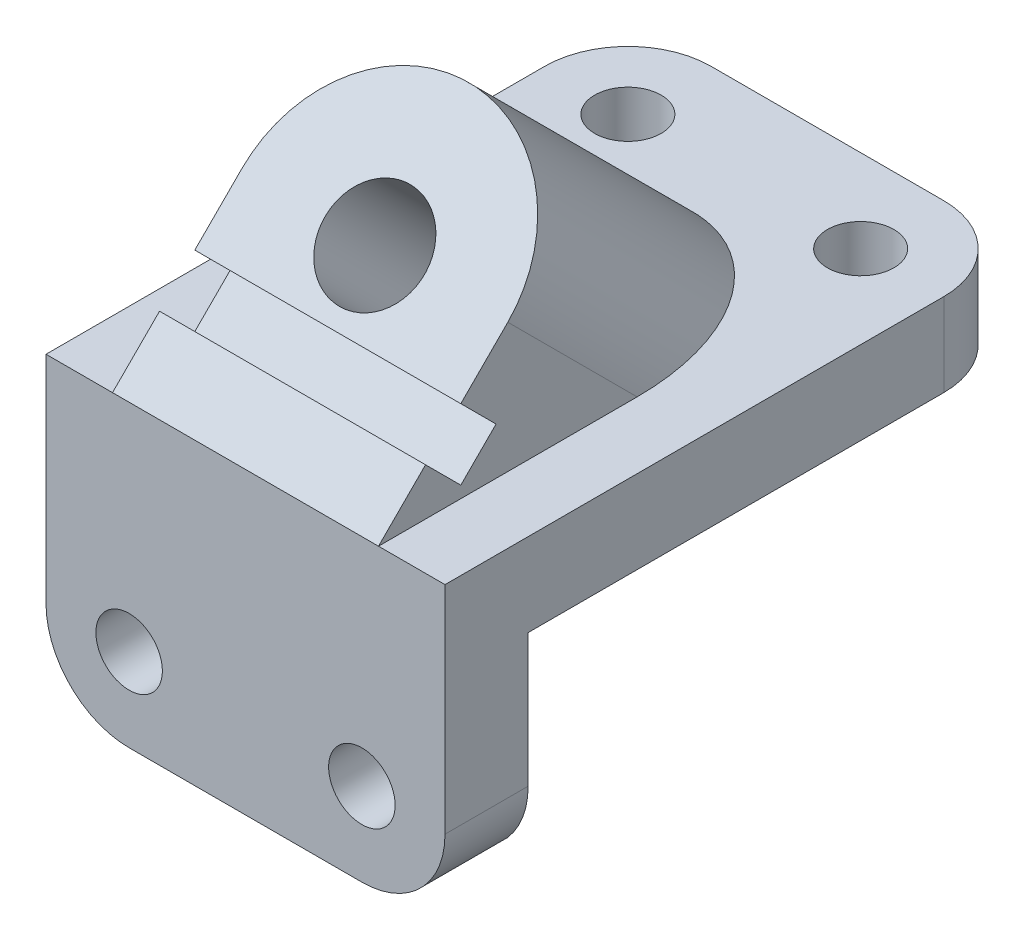
ISO-10303-21;
HEADER;
FILE_DESCRIPTION(('STEP AP214'),'2;1');
FILE_NAME('part.step','',(''),(''),'','','');
FILE_SCHEMA(('AUTOMOTIVE_DESIGN { 1 0 10303 214 1 1 1 1 }'));
ENDSEC;
DATA;
#1=APPLICATION_CONTEXT('core data for automotive mechanical design processes');
#2=APPLICATION_PROTOCOL_DEFINITION('international standard','automotive_design',2000,#1);
#3=PRODUCT_CONTEXT('',#1,'mechanical');
#4=PRODUCT('Part','Part','',(#3));
#5=PRODUCT_RELATED_PRODUCT_CATEGORY('part','',(#4));
#6=PRODUCT_DEFINITION_FORMATION('','',#4);
#7=PRODUCT_DEFINITION_CONTEXT('part definition',#1,'design');
#8=PRODUCT_DEFINITION('design','',#6,#7);
#9=PRODUCT_DEFINITION_SHAPE('','',#8);
#10=(LENGTH_UNIT() NAMED_UNIT(*) SI_UNIT(.MILLI.,.METRE.));
#11=(NAMED_UNIT(*) PLANE_ANGLE_UNIT() SI_UNIT($,.RADIAN.));
#12=(NAMED_UNIT(*) SI_UNIT($,.STERADIAN.) SOLID_ANGLE_UNIT());
#13=UNCERTAINTY_MEASURE_WITH_UNIT(LENGTH_MEASURE(1.E-05),#10,'distance_accuracy_value','');
#14=(GEOMETRIC_REPRESENTATION_CONTEXT(3) GLOBAL_UNCERTAINTY_ASSIGNED_CONTEXT((#13)) GLOBAL_UNIT_ASSIGNED_CONTEXT((#10,
#11,#12)) REPRESENTATION_CONTEXT('',''));
#15=CARTESIAN_POINT('',(0.,0.,0.));
#16=DIRECTION('',(0.,0.,1.));
#17=DIRECTION('',(1.,0.,0.));
#18=AXIS2_PLACEMENT_3D('',#15,#16,#17);
#19=CARTESIAN_POINT('',(60.,112.175144212722,-67.1751442127221));
#20=DIRECTION('',(0.,-0.707106781186549,-0.707106781186547));
#21=DIRECTION('',(0.,0.707106781186547,-0.707106781186549));
#22=AXIS2_PLACEMENT_3D('',#19,#20,#21);
#23=PLANE('',#22);
#24=CARTESIAN_POINT('',(0.,83.8908729652601,-38.8908729652602));
#25=DIRECTION('',(0.,0.707106781186548,0.707106781186547));
#26=DIRECTION('',(0.,-0.707106781186547,0.707106781186548));
#27=AXIS2_PLACEMENT_3D('',#24,#25,#26);
#28=CIRCLE('',#27,15.);
#29=CARTESIAN_POINT('',(0.,73.2842712474619,-28.2842712474619));
#30=VERTEX_POINT('',#29);
#31=EDGE_CURVE('E256',#30,#30,#28,.T.);
#32=ORIENTED_EDGE('',*,*,#31,.F.);
#33=EDGE_LOOP('',(#32));
#34=FACE_BOUND('',#33,.T.);
#35=DIRECTION('',(0.,-0.707106781186547,0.707106781186548));
#36=VECTOR('',#35,1.);
#37=CARTESIAN_POINT('',(-40.,22.5000000000001,22.5));
#38=LINE('',#37,#36);
#39=CARTESIAN_POINT('',(-40.,83.8908729652601,-38.8908729652602));
#40=VERTEX_POINT('',#39);
#41=CARTESIAN_POINT('',(-40.,69.7487373415292,-24.7487373415292));
#42=VERTEX_POINT('',#41);
#43=EDGE_CURVE('E284',#40,#42,#38,.T.);
#44=ORIENTED_EDGE('',*,*,#43,.T.);
#45=DIRECTION('',(-1.,0.,0.));
#46=VECTOR('',#45,1.);
#47=CARTESIAN_POINT('',(-40.,69.7487373415292,-24.7487373415292));
#48=LINE('',#47,#46);
#49=CARTESIAN_POINT('',(40.,69.7487373415292,-24.7487373415292));
#50=VERTEX_POINT('',#49);
#51=EDGE_CURVE('E242',#50,#42,#48,.T.);
#52=ORIENTED_EDGE('',*,*,#51,.F.);
#53=DIRECTION('',(0.,0.707106781186547,-0.707106781186548));
#54=VECTOR('',#53,1.);
#55=CARTESIAN_POINT('',(40.,22.5000000000001,22.5));
#56=LINE('',#55,#54);
#57=CARTESIAN_POINT('',(40.,83.8908729652601,-38.8908729652602));
#58=VERTEX_POINT('',#57);
#59=EDGE_CURVE('E263',#50,#58,#56,.T.);
#60=ORIENTED_EDGE('',*,*,#59,.T.);
#61=CARTESIAN_POINT('',(0.,83.8908729652601,-38.8908729652602));
#62=DIRECTION('',(0.,0.707106781186548,0.707106781186547));
#63=DIRECTION('',(0.,-0.707106781186547,0.707106781186548));
#64=AXIS2_PLACEMENT_3D('',#61,#62,#63);
#65=CIRCLE('',#64,40.);
#66=EDGE_CURVE('E268',#58,#40,#65,.T.);
#67=ORIENTED_EDGE('',*,*,#66,.T.);
#68=EDGE_LOOP('',(#44,#52,#60,#67));
#69=FACE_BOUND('',#68,.T.);
#70=ADVANCED_FACE('F110',(#34,#69),#23,.F.);
#71=CARTESIAN_POINT('',(40.,45.,0.));
#72=VERTEX_POINT('',#71);
#73=CARTESIAN_POINT('',(40.,59.142135623731,-14.142135623731));
#74=VERTEX_POINT('',#73);
#75=EDGE_CURVE('E266',#72,#74,#56,.T.);
#76=ORIENTED_EDGE('',*,*,#75,.T.);
#77=DIRECTION('',(1.,0.,0.));
#78=VECTOR('',#77,1.);
#79=CARTESIAN_POINT('',(40.,59.142135623731,-14.142135623731));
#80=LINE('',#79,#78);
#81=CARTESIAN_POINT('',(-40.,59.1421356237309,-14.142135623731));
#82=VERTEX_POINT('',#81);
#83=EDGE_CURVE('E626',#82,#74,#80,.T.);
#84=ORIENTED_EDGE('',*,*,#83,.F.);
#85=CARTESIAN_POINT('',(-40.,45.,0.));
#86=VERTEX_POINT('',#85);
#87=EDGE_CURVE('E248',#82,#86,#38,.T.);
#88=ORIENTED_EDGE('',*,*,#87,.T.);
#89=DIRECTION('',(-1.,0.,0.));
#90=VECTOR('',#89,1.);
#91=CARTESIAN_POINT('',(-60.,45.,0.));
#92=LINE('',#91,#90);
#93=EDGE_CURVE('E353',#72,#86,#92,.T.);
#94=ORIENTED_EDGE('',*,*,#93,.F.);
#95=EDGE_LOOP('',(#76,#84,#88,#94));
#96=FACE_BOUND('',#95,.T.);
#97=ADVANCED_FACE('F457',(#96),#23,.F.);
#98=CARTESIAN_POINT('',(60.,45.,-25.));
#99=DIRECTION('',(1.,0.,0.));
#100=DIRECTION('',(0.,1.,0.));
#101=AXIS2_PLACEMENT_3D('',#98,#99,#100);
#102=PLANE('',#101);
#103=DIRECTION('',(0.,0.,1.));
#104=VECTOR('',#103,1.);
#105=CARTESIAN_POINT('',(60.,45.,-25.));
#106=LINE('',#105,#104);
#107=CARTESIAN_POINT('',(60.,45.,-150.));
#108=VERTEX_POINT('',#107);
#109=CARTESIAN_POINT('',(60.,45.,0.));
#110=VERTEX_POINT('',#109);
#111=EDGE_CURVE('E357',#108,#110,#106,.T.);
#112=ORIENTED_EDGE('',*,*,#111,.T.);
#113=DIRECTION('',(0.,1.,0.));
#114=VECTOR('',#113,1.);
#115=CARTESIAN_POINT('',(60.,45.,0.));
#116=LINE('',#115,#114);
#117=CARTESIAN_POINT('',(60.,-19.9999999999998,0.));
#118=VERTEX_POINT('',#117);
#119=EDGE_CURVE('E348',#118,#110,#116,.T.);
#120=ORIENTED_EDGE('',*,*,#119,.F.);
#121=DIRECTION('',(0.,0.,1.));
#122=VECTOR('',#121,1.);
#123=CARTESIAN_POINT('',(60.,-19.9999999999998,-25.));
#124=LINE('',#123,#122);
#125=CARTESIAN_POINT('',(60.,-19.9999999999998,-25.));
#126=VERTEX_POINT('',#125);
#127=EDGE_CURVE('E360',#126,#118,#124,.T.);
#128=ORIENTED_EDGE('',*,*,#127,.F.);
#129=DIRECTION('',(0.,1.,0.));
#130=VECTOR('',#129,1.);
#131=CARTESIAN_POINT('',(60.,45.,-25.));
#132=LINE('',#131,#130);
#133=CARTESIAN_POINT('',(60.,20.,-25.));
#134=VERTEX_POINT('',#133);
#135=EDGE_CURVE('E331',#126,#134,#132,.T.);
#136=ORIENTED_EDGE('',*,*,#135,.T.);
#137=DIRECTION('',(0.,0.,-1.));
#138=VECTOR('',#137,1.);
#139=CARTESIAN_POINT('',(60.,20.,-175.));
#140=LINE('',#139,#138);
#141=CARTESIAN_POINT('',(60.,20.,-150.));
#142=VERTEX_POINT('',#141);
#143=EDGE_CURVE('E299',#134,#142,#140,.T.);
#144=ORIENTED_EDGE('',*,*,#143,.T.);
#145=DIRECTION('',(0.,1.,0.));
#146=VECTOR('',#145,1.);
#147=CARTESIAN_POINT('',(60.,45.,-150.));
#148=LINE('',#147,#146);
#149=EDGE_CURVE('E12',#142,#108,#148,.T.);
#150=ORIENTED_EDGE('',*,*,#149,.T.);
#151=EDGE_LOOP('',(#112,#120,#128,#136,#144,#150));
#152=FACE_BOUND('',#151,.T.);
#153=ADVANCED_FACE('F413',(#152),#102,.T.);
#154=CARTESIAN_POINT('',(-60.,45.,-25.));
#155=DIRECTION('',(-1.,0.,0.));
#156=DIRECTION('',(0.,-1.,0.));
#157=AXIS2_PLACEMENT_3D('',#154,#155,#156);
#158=PLANE('',#157);
#159=DIRECTION('',(0.,-1.,0.));
#160=VECTOR('',#159,1.);
#161=CARTESIAN_POINT('',(-60.,45.,0.));
#162=LINE('',#161,#160);
#163=CARTESIAN_POINT('',(-60.,45.,0.));
#164=VERTEX_POINT('',#163);
#165=CARTESIAN_POINT('',(-60.,-20.,0.));
#166=VERTEX_POINT('',#165);
#167=EDGE_CURVE('E319',#164,#166,#162,.T.);
#168=ORIENTED_EDGE('',*,*,#167,.F.);
#169=DIRECTION('',(0.,0.,1.));
#170=VECTOR('',#169,1.);
#171=CARTESIAN_POINT('',(-60.,45.,-25.));
#172=LINE('',#171,#170);
#173=CARTESIAN_POINT('',(-60.,45.,-150.));
#174=VERTEX_POINT('',#173);
#175=EDGE_CURVE('E352',#174,#164,#172,.T.);
#176=ORIENTED_EDGE('',*,*,#175,.F.);
#177=DIRECTION('',(0.,1.,0.));
#178=VECTOR('',#177,1.);
#179=CARTESIAN_POINT('',(-60.,45.,-150.));
#180=LINE('',#179,#178);
#181=CARTESIAN_POINT('',(-60.,20.,-150.));
#182=VERTEX_POINT('',#181);
#183=EDGE_CURVE('E372',#174,#182,#180,.F.);
#184=ORIENTED_EDGE('',*,*,#183,.T.);
#185=DIRECTION('',(0.,0.,-1.));
#186=VECTOR('',#185,1.);
#187=CARTESIAN_POINT('',(-60.,20.,-175.));
#188=LINE('',#187,#186);
#189=CARTESIAN_POINT('',(-60.,19.9999999999999,-25.));
#190=VERTEX_POINT('',#189);
#191=EDGE_CURVE('E294',#190,#182,#188,.T.);
#192=ORIENTED_EDGE('',*,*,#191,.F.);
#193=DIRECTION('',(0.,-1.,0.));
#194=VECTOR('',#193,1.);
#195=CARTESIAN_POINT('',(-60.,45.,-25.));
#196=LINE('',#195,#194);
#197=CARTESIAN_POINT('',(-60.,-20.,-25.));
#198=VERTEX_POINT('',#197);
#199=EDGE_CURVE('E322',#190,#198,#196,.T.);
#200=ORIENTED_EDGE('',*,*,#199,.T.);
#201=DIRECTION('',(0.,0.,1.));
#202=VECTOR('',#201,1.);
#203=CARTESIAN_POINT('',(-60.,-20.,-25.));
#204=LINE('',#203,#202);
#205=EDGE_CURVE('E337',#198,#166,#204,.T.);
#206=ORIENTED_EDGE('',*,*,#205,.T.);
#207=EDGE_LOOP('',(#168,#176,#184,#192,#200,#206));
#208=FACE_BOUND('',#207,.T.);
#209=ADVANCED_FACE('F421',(#208),#158,.T.);
#210=CARTESIAN_POINT('',(-35.,-20.,-25.));
#211=DIRECTION('',(0.,0.,-1.));
#212=DIRECTION('',(-1.,0.,0.));
#213=AXIS2_PLACEMENT_3D('',#210,#211,#212);
#214=PLANE('',#213);
#215=CARTESIAN_POINT('',(35.,-20.,-25.));
#216=DIRECTION('',(0.,0.,1.));
#217=DIRECTION('',(1.,0.,0.));
#218=AXIS2_PLACEMENT_3D('',#215,#216,#217);
#219=CIRCLE('',#218,10.);
#220=CARTESIAN_POINT('',(45.,-20.,-25.));
#221=VERTEX_POINT('',#220);
#222=EDGE_CURVE('E307',#221,#221,#219,.T.);
#223=ORIENTED_EDGE('',*,*,#222,.T.);
#224=EDGE_LOOP('',(#223));
#225=FACE_BOUND('',#224,.T.);
#226=CARTESIAN_POINT('',(-35.,-20.,-25.));
#227=DIRECTION('',(0.,0.,1.));
#228=DIRECTION('',(1.,0.,0.));
#229=AXIS2_PLACEMENT_3D('',#226,#227,#228);
#230=CIRCLE('',#229,10.);
#231=CARTESIAN_POINT('',(-25.,-20.,-25.));
#232=VERTEX_POINT('',#231);
#233=EDGE_CURVE('E314',#232,#232,#230,.T.);
#234=ORIENTED_EDGE('',*,*,#233,.T.);
#235=EDGE_LOOP('',(#234));
#236=FACE_BOUND('',#235,.T.);
#237=ORIENTED_EDGE('',*,*,#199,.F.);
#238=DIRECTION('',(1.,0.,0.));
#239=VECTOR('',#238,1.);
#240=CARTESIAN_POINT('',(-60.,19.9999999999999,-25.));
#241=LINE('',#240,#239);
#242=EDGE_CURVE('E296',#190,#134,#241,.T.);
#243=ORIENTED_EDGE('',*,*,#242,.T.);
#244=ORIENTED_EDGE('',*,*,#135,.F.);
#245=CARTESIAN_POINT('',(35.,-20.,-25.));
#246=DIRECTION('',(0.,0.,1.));
#247=DIRECTION('',(-1.,0.,0.));
#248=AXIS2_PLACEMENT_3D('',#245,#246,#247);
#249=CIRCLE('',#248,25.);
#250=CARTESIAN_POINT('',(34.9999999999998,-45.,-25.));
#251=VERTEX_POINT('',#250);
#252=EDGE_CURVE('E329',#251,#126,#249,.T.);
#253=ORIENTED_EDGE('',*,*,#252,.F.);
#254=DIRECTION('',(1.,0.,0.));
#255=VECTOR('',#254,1.);
#256=CARTESIAN_POINT('',(-34.9999999999998,-45.,-25.));
#257=LINE('',#256,#255);
#258=CARTESIAN_POINT('',(-34.9999999999998,-45.,-25.));
#259=VERTEX_POINT('',#258);
#260=EDGE_CURVE('E330',#259,#251,#257,.T.);
#261=ORIENTED_EDGE('',*,*,#260,.F.);
#262=CARTESIAN_POINT('',(-35.,-20.,-25.));
#263=DIRECTION('',(0.,0.,1.));
#264=DIRECTION('',(-1.,0.,0.));
#265=AXIS2_PLACEMENT_3D('',#262,#263,#264);
#266=CIRCLE('',#265,25.);
#267=EDGE_CURVE('E324',#198,#259,#266,.T.);
#268=ORIENTED_EDGE('',*,*,#267,.F.);
#269=EDGE_LOOP('',(#237,#243,#244,#253,#261,#268));
#270=FACE_BOUND('',#269,.T.);
#271=ADVANCED_FACE('F420',(#225,#236,#270),#214,.T.);
#272=CARTESIAN_POINT('',(-60.,45.,-25.));
#273=DIRECTION('',(0.,1.,0.));
#274=DIRECTION('',(0.,0.,1.));
#275=AXIS2_PLACEMENT_3D('',#272,#273,#274);
#276=PLANE('',#275);
#277=CARTESIAN_POINT('',(0.,45.,-77.7817459305201));
#278=DIRECTION('',(0.,1.,0.));
#279=DIRECTION('',(0.,0.,1.));
#280=AXIS2_PLACEMENT_3D('',#277,#278,#279);
#281=ELLIPSE('',#280,56.5685424949237,40.);
#282=CARTESIAN_POINT('',(-40.,45.,-77.7817459305201));
#283=VERTEX_POINT('',#282);
#284=CARTESIAN_POINT('',(40.,45.,-77.7817459305201));
#285=VERTEX_POINT('',#284);
#286=EDGE_CURVE('E271',#283,#285,#281,.F.);
#287=ORIENTED_EDGE('',*,*,#286,.T.);
#288=DIRECTION('',(0.,0.,1.));
#289=VECTOR('',#288,1.);
#290=CARTESIAN_POINT('',(40.,45.,-106.993706197148));
#291=LINE('',#290,#289);
#292=EDGE_CURVE('E262',#285,#72,#291,.T.);
#293=ORIENTED_EDGE('',*,*,#292,.T.);
#294=EDGE_CURVE('E321',#110,#72,#92,.T.);
#295=ORIENTED_EDGE('',*,*,#294,.F.);
#296=ORIENTED_EDGE('',*,*,#111,.F.);
#297=CARTESIAN_POINT('',(35.,45.,-150.));
#298=DIRECTION('',(0.,1.,0.));
#299=DIRECTION('',(0.,0.,1.));
#300=AXIS2_PLACEMENT_3D('',#297,#298,#299);
#301=CIRCLE('',#300,25.);
#302=CARTESIAN_POINT('',(35.,45.,-175.));
#303=VERTEX_POINT('',#302);
#304=EDGE_CURVE('E369',#108,#303,#301,.T.);
#305=ORIENTED_EDGE('',*,*,#304,.T.);
#306=DIRECTION('',(1.,0.,0.));
#307=VECTOR('',#306,1.);
#308=CARTESIAN_POINT('',(-60.,45.,-175.));
#309=LINE('',#308,#307);
#310=CARTESIAN_POINT('',(-35.,45.,-175.));
#311=VERTEX_POINT('',#310);
#312=EDGE_CURVE('E301',#311,#303,#309,.T.);
#313=ORIENTED_EDGE('',*,*,#312,.F.);
#314=CARTESIAN_POINT('',(-35.,45.,-150.));
#315=DIRECTION('',(0.,1.,0.));
#316=DIRECTION('',(0.,0.,1.));
#317=AXIS2_PLACEMENT_3D('',#314,#315,#316);
#318=CIRCLE('',#317,25.);
#319=EDGE_CURVE('E375',#311,#174,#318,.T.);
#320=ORIENTED_EDGE('',*,*,#319,.T.);
#321=ORIENTED_EDGE('',*,*,#175,.T.);
#322=DIRECTION('',(1.,0.,0.));
#323=VECTOR('',#322,1.);
#324=CARTESIAN_POINT('',(0.,45.,0.));
#325=LINE('',#324,#323);
#326=EDGE_CURVE('E285',#164,#86,#325,.T.);
#327=ORIENTED_EDGE('',*,*,#326,.T.);
#328=DIRECTION('',(0.,0.,-1.));
#329=VECTOR('',#328,1.);
#330=CARTESIAN_POINT('',(-40.,45.,-106.993706197148));
#331=LINE('',#330,#329);
#332=EDGE_CURVE('E277',#86,#283,#331,.T.);
#333=ORIENTED_EDGE('',*,*,#332,.T.);
#334=EDGE_LOOP('',(#287,#293,#295,#296,#305,#313,#320,#321,#327,#333));
#335=FACE_BOUND('',#334,.T.);
#336=CARTESIAN_POINT('',(35.,45.,-150.));
#337=DIRECTION('',(0.,1.,0.));
#338=DIRECTION('',(0.,0.,1.));
#339=AXIS2_PLACEMENT_3D('',#336,#337,#338);
#340=CIRCLE('',#339,10.);
#341=CARTESIAN_POINT('',(35.,45.,-140.));
#342=VERTEX_POINT('',#341);
#343=EDGE_CURVE('E287',#342,#342,#340,.T.);
#344=ORIENTED_EDGE('',*,*,#343,.F.);
#345=EDGE_LOOP('',(#344));
#346=FACE_BOUND('',#345,.T.);
#347=CARTESIAN_POINT('',(-35.,45.,-150.));
#348=DIRECTION('',(0.,1.,0.));
#349=DIRECTION('',(0.,0.,1.));
#350=AXIS2_PLACEMENT_3D('',#347,#348,#349);
#351=CIRCLE('',#350,10.);
#352=CARTESIAN_POINT('',(-35.,45.,-140.));
#353=VERTEX_POINT('',#352);
#354=EDGE_CURVE('E273',#353,#353,#351,.T.);
#355=ORIENTED_EDGE('',*,*,#354,.F.);
#356=EDGE_LOOP('',(#355));
#357=FACE_BOUND('',#356,.T.);
#358=ADVANCED_FACE('F403',(#335,#346,#357),#276,.T.);
#359=CARTESIAN_POINT('',(35.,-20.,-25.));
#360=DIRECTION('',(0.,0.,1.));
#361=DIRECTION('',(1.,0.,0.));
#362=AXIS2_PLACEMENT_3D('',#359,#360,#361);
#363=CYLINDRICAL_SURFACE('',#362,25.);
#364=CARTESIAN_POINT('',(35.,-20.,0.));
#365=DIRECTION('',(0.,0.,1.));
#366=DIRECTION('',(-1.,0.,0.));
#367=AXIS2_PLACEMENT_3D('',#364,#365,#366);
#368=CIRCLE('',#367,25.);
#369=CARTESIAN_POINT('',(34.9999999999998,-45.,0.));
#370=VERTEX_POINT('',#369);
#371=EDGE_CURVE('E343',#370,#118,#368,.T.);
#372=ORIENTED_EDGE('',*,*,#371,.F.);
#373=DIRECTION('',(0.,0.,1.));
#374=VECTOR('',#373,1.);
#375=CARTESIAN_POINT('',(34.9999999999998,-45.,-25.));
#376=LINE('',#375,#374);
#377=EDGE_CURVE('E363',#251,#370,#376,.T.);
#378=ORIENTED_EDGE('',*,*,#377,.F.);
#379=ORIENTED_EDGE('',*,*,#252,.T.);
#380=ORIENTED_EDGE('',*,*,#127,.T.);
#381=EDGE_LOOP('',(#372,#378,#379,#380));
#382=FACE_BOUND('',#381,.T.);
#383=ADVANCED_FACE('F450',(#382),#363,.T.);
#384=CARTESIAN_POINT('',(-34.9999999999998,-45.,-25.));
#385=DIRECTION('',(0.,-1.,0.));
#386=DIRECTION('',(0.,0.,-1.));
#387=AXIS2_PLACEMENT_3D('',#384,#385,#386);
#388=PLANE('',#387);
#389=DIRECTION('',(1.,0.,0.));
#390=VECTOR('',#389,1.);
#391=CARTESIAN_POINT('',(-34.9999999999998,-45.,0.));
#392=LINE('',#391,#390);
#393=CARTESIAN_POINT('',(-34.9999999999998,-45.,0.));
#394=VERTEX_POINT('',#393);
#395=EDGE_CURVE('E345',#394,#370,#392,.T.);
#396=ORIENTED_EDGE('',*,*,#395,.F.);
#397=DIRECTION('',(0.,0.,1.));
#398=VECTOR('',#397,1.);
#399=CARTESIAN_POINT('',(-34.9999999999998,-45.,-25.));
#400=LINE('',#399,#398);
#401=EDGE_CURVE('E361',#259,#394,#400,.T.);
#402=ORIENTED_EDGE('',*,*,#401,.F.);
#403=ORIENTED_EDGE('',*,*,#260,.T.);
#404=ORIENTED_EDGE('',*,*,#377,.T.);
#405=EDGE_LOOP('',(#396,#402,#403,#404));
#406=FACE_BOUND('',#405,.T.);
#407=ADVANCED_FACE('F446',(#406),#388,.T.);
#408=CARTESIAN_POINT('',(-35.,-20.,-25.));
#409=DIRECTION('',(0.,0.,1.));
#410=DIRECTION('',(1.,0.,0.));
#411=AXIS2_PLACEMENT_3D('',#408,#409,#410);
#412=CYLINDRICAL_SURFACE('',#411,25.);
#413=CARTESIAN_POINT('',(-35.,-20.,0.));
#414=DIRECTION('',(0.,0.,1.));
#415=DIRECTION('',(-1.,0.,0.));
#416=AXIS2_PLACEMENT_3D('',#413,#414,#415);
#417=CIRCLE('',#416,25.);
#418=EDGE_CURVE('E339',#166,#394,#417,.T.);
#419=ORIENTED_EDGE('',*,*,#418,.F.);
#420=ORIENTED_EDGE('',*,*,#205,.F.);
#421=ORIENTED_EDGE('',*,*,#267,.T.);
#422=ORIENTED_EDGE('',*,*,#401,.T.);
#423=EDGE_LOOP('',(#419,#420,#421,#422));
#424=FACE_BOUND('',#423,.T.);
#425=ADVANCED_FACE('F428',(#424),#412,.T.);
#426=CARTESIAN_POINT('',(-35.,-20.,0.));
#427=DIRECTION('',(0.,0.,-1.));
#428=DIRECTION('',(-1.,0.,0.));
#429=AXIS2_PLACEMENT_3D('',#426,#427,#428);
#430=PLANE('',#429);
#431=CARTESIAN_POINT('',(35.,-20.,0.));
#432=DIRECTION('',(0.,0.,1.));
#433=DIRECTION('',(1.,0.,0.));
#434=AXIS2_PLACEMENT_3D('',#431,#432,#433);
#435=CIRCLE('',#434,10.);
#436=CARTESIAN_POINT('',(45.,-20.,0.));
#437=VERTEX_POINT('',#436);
#438=EDGE_CURVE('E302',#437,#437,#435,.T.);
#439=ORIENTED_EDGE('',*,*,#438,.F.);
#440=EDGE_LOOP('',(#439));
#441=FACE_BOUND('',#440,.T.);
#442=CARTESIAN_POINT('',(-35.,-20.,0.));
#443=DIRECTION('',(0.,0.,1.));
#444=DIRECTION('',(1.,0.,0.));
#445=AXIS2_PLACEMENT_3D('',#442,#443,#444);
#446=CIRCLE('',#445,10.);
#447=CARTESIAN_POINT('',(-25.,-20.,0.));
#448=VERTEX_POINT('',#447);
#449=EDGE_CURVE('E315',#448,#448,#446,.T.);
#450=ORIENTED_EDGE('',*,*,#449,.F.);
#451=EDGE_LOOP('',(#450));
#452=FACE_BOUND('',#451,.T.);
#453=ORIENTED_EDGE('',*,*,#167,.T.);
#454=ORIENTED_EDGE('',*,*,#418,.T.);
#455=ORIENTED_EDGE('',*,*,#395,.T.);
#456=ORIENTED_EDGE('',*,*,#371,.T.);
#457=ORIENTED_EDGE('',*,*,#119,.T.);
#458=ORIENTED_EDGE('',*,*,#294,.T.);
#459=ORIENTED_EDGE('',*,*,#93,.T.);
#460=ORIENTED_EDGE('',*,*,#326,.F.);
#461=EDGE_LOOP('',(#453,#454,#455,#456,#457,#458,#459,#460));
#462=FACE_BOUND('',#461,.T.);
#463=ADVANCED_FACE('F427',(#441,#452,#462),#430,.F.);
#464=CARTESIAN_POINT('',(-35.,-20.,-25.));
#465=DIRECTION('',(0.,0.,1.));
#466=DIRECTION('',(1.,0.,0.));
#467=AXIS2_PLACEMENT_3D('',#464,#465,#466);
#468=CYLINDRICAL_SURFACE('',#467,10.);
#469=ORIENTED_EDGE('',*,*,#233,.F.);
#470=EDGE_LOOP('',(#469));
#471=FACE_BOUND('',#470,.T.);
#472=ORIENTED_EDGE('',*,*,#449,.T.);
#473=EDGE_LOOP('',(#472));
#474=FACE_BOUND('',#473,.T.);
#475=ADVANCED_FACE('F485',(#471,#474),#468,.F.);
#476=CARTESIAN_POINT('',(35.,-20.,-25.));
#477=DIRECTION('',(0.,0.,1.));
#478=DIRECTION('',(1.,0.,0.));
#479=AXIS2_PLACEMENT_3D('',#476,#477,#478);
#480=CYLINDRICAL_SURFACE('',#479,10.);
#481=ORIENTED_EDGE('',*,*,#222,.F.);
#482=EDGE_LOOP('',(#481));
#483=FACE_BOUND('',#482,.T.);
#484=ORIENTED_EDGE('',*,*,#438,.T.);
#485=EDGE_LOOP('',(#484));
#486=FACE_BOUND('',#485,.T.);
#487=ADVANCED_FACE('F478',(#483,#486),#480,.F.);
#488=CARTESIAN_POINT('',(-60.,45.,-175.));
#489=DIRECTION('',(0.,0.,-1.));
#490=DIRECTION('',(-1.,0.,0.));
#491=AXIS2_PLACEMENT_3D('',#488,#489,#490);
#492=PLANE('',#491);
#493=DIRECTION('',(1.,0.,0.));
#494=VECTOR('',#493,1.);
#495=CARTESIAN_POINT('',(-60.,20.,-175.));
#496=LINE('',#495,#494);
#497=CARTESIAN_POINT('',(-35.,20.,-175.));
#498=VERTEX_POINT('',#497);
#499=CARTESIAN_POINT('',(35.,20.,-175.));
#500=VERTEX_POINT('',#499);
#501=EDGE_CURVE('E304',#498,#500,#496,.T.);
#502=ORIENTED_EDGE('',*,*,#501,.F.);
#503=DIRECTION('',(0.,1.,0.));
#504=VECTOR('',#503,1.);
#505=CARTESIAN_POINT('',(-35.,45.,-175.));
#506=LINE('',#505,#504);
#507=EDGE_CURVE('E370',#498,#311,#506,.T.);
#508=ORIENTED_EDGE('',*,*,#507,.T.);
#509=ORIENTED_EDGE('',*,*,#312,.T.);
#510=DIRECTION('',(0.,1.,0.));
#511=VECTOR('',#510,1.);
#512=CARTESIAN_POINT('',(35.,45.,-175.));
#513=LINE('',#512,#511);
#514=EDGE_CURVE('E358',#303,#500,#513,.F.);
#515=ORIENTED_EDGE('',*,*,#514,.T.);
#516=EDGE_LOOP('',(#502,#508,#509,#515));
#517=FACE_BOUND('',#516,.T.);
#518=ADVANCED_FACE('F388',(#517),#492,.T.);
#519=CARTESIAN_POINT('',(-60.,20.,-175.));
#520=DIRECTION('',(0.,-1.,0.));
#521=DIRECTION('',(1.,0.,0.));
#522=AXIS2_PLACEMENT_3D('',#519,#520,#521);
#523=PLANE('',#522);
#524=CARTESIAN_POINT('',(0.,20.,-102.78174593052));
#525=DIRECTION('',(0.,-1.,0.));
#526=DIRECTION('',(0.,0.,1.));
#527=AXIS2_PLACEMENT_3D('',#524,#525,#526);
#528=ELLIPSE('',#527,21.2132034355964,15.);
#529=CARTESIAN_POINT('',(0.,20.,-81.5685424949237));
#530=VERTEX_POINT('',#529);
#531=EDGE_CURVE('E257',#530,#530,#528,.T.);
#532=ORIENTED_EDGE('',*,*,#531,.F.);
#533=EDGE_LOOP('',(#532));
#534=FACE_BOUND('',#533,.T.);
#535=CARTESIAN_POINT('',(35.,20.,-150.));
#536=DIRECTION('',(0.,-1.,0.));
#537=DIRECTION('',(1.,0.,0.));
#538=AXIS2_PLACEMENT_3D('',#535,#536,#537);
#539=CIRCLE('',#538,10.);
#540=CARTESIAN_POINT('',(35.,20.,-140.));
#541=VERTEX_POINT('',#540);
#542=EDGE_CURVE('E111',#541,#541,#539,.T.);
#543=ORIENTED_EDGE('',*,*,#542,.F.);
#544=EDGE_LOOP('',(#543));
#545=FACE_BOUND('',#544,.T.);
#546=CARTESIAN_POINT('',(-35.,20.,-150.));
#547=DIRECTION('',(0.,-1.,0.));
#548=DIRECTION('',(1.,0.,0.));
#549=AXIS2_PLACEMENT_3D('',#546,#547,#548);
#550=CIRCLE('',#549,10.);
#551=CARTESIAN_POINT('',(-35.,20.,-140.));
#552=VERTEX_POINT('',#551);
#553=EDGE_CURVE('E292',#552,#552,#550,.T.);
#554=ORIENTED_EDGE('',*,*,#553,.F.);
#555=EDGE_LOOP('',(#554));
#556=FACE_BOUND('',#555,.T.);
#557=ORIENTED_EDGE('',*,*,#191,.T.);
#558=CARTESIAN_POINT('',(-35.,20.,-150.));
#559=DIRECTION('',(0.,-1.,0.));
#560=DIRECTION('',(1.,0.,0.));
#561=AXIS2_PLACEMENT_3D('',#558,#559,#560);
#562=CIRCLE('',#561,25.);
#563=EDGE_CURVE('E116',#182,#498,#562,.T.);
#564=ORIENTED_EDGE('',*,*,#563,.T.);
#565=ORIENTED_EDGE('',*,*,#501,.T.);
#566=CARTESIAN_POINT('',(35.,20.,-150.));
#567=DIRECTION('',(0.,-1.,0.));
#568=DIRECTION('',(1.,0.,0.));
#569=AXIS2_PLACEMENT_3D('',#566,#567,#568);
#570=CIRCLE('',#569,25.);
#571=EDGE_CURVE('E135',#500,#142,#570,.T.);
#572=ORIENTED_EDGE('',*,*,#571,.T.);
#573=ORIENTED_EDGE('',*,*,#143,.F.);
#574=ORIENTED_EDGE('',*,*,#242,.F.);
#575=EDGE_LOOP('',(#557,#564,#565,#572,#573,#574));
#576=FACE_BOUND('',#575,.T.);
#577=ADVANCED_FACE('F387',(#534,#545,#556,#576),#523,.T.);
#578=CARTESIAN_POINT('',(-35.,45.,-150.));
#579=DIRECTION('',(0.,1.,0.));
#580=DIRECTION('',(-1.,0.,0.));
#581=AXIS2_PLACEMENT_3D('',#578,#579,#580);
#582=CYLINDRICAL_SURFACE('',#581,25.);
#583=ORIENTED_EDGE('',*,*,#563,.F.);
#584=ORIENTED_EDGE('',*,*,#183,.F.);
#585=ORIENTED_EDGE('',*,*,#319,.F.);
#586=ORIENTED_EDGE('',*,*,#507,.F.);
#587=EDGE_LOOP('',(#583,#584,#585,#586));
#588=FACE_BOUND('',#587,.T.);
#589=ADVANCED_FACE('F386',(#588),#582,.T.);
#590=CARTESIAN_POINT('',(35.,45.,-150.));
#591=DIRECTION('',(0.,1.,0.));
#592=DIRECTION('',(-1.,0.,0.));
#593=AXIS2_PLACEMENT_3D('',#590,#591,#592);
#594=CYLINDRICAL_SURFACE('',#593,25.);
#595=ORIENTED_EDGE('',*,*,#571,.F.);
#596=ORIENTED_EDGE('',*,*,#514,.F.);
#597=ORIENTED_EDGE('',*,*,#304,.F.);
#598=ORIENTED_EDGE('',*,*,#149,.F.);
#599=EDGE_LOOP('',(#595,#596,#597,#598));
#600=FACE_BOUND('',#599,.T.);
#601=ADVANCED_FACE('F107',(#600),#594,.T.);
#602=CARTESIAN_POINT('',(-35.,-45.,-150.));
#603=DIRECTION('',(0.,1.,0.));
#604=DIRECTION('',(0.,0.,1.));
#605=AXIS2_PLACEMENT_3D('',#602,#603,#604);
#606=CYLINDRICAL_SURFACE('',#605,10.);
#607=CARTESIAN_POINT('',(-35.,20.,-140.));
#608=CARTESIAN_POINT('',(-35.,20.2604166666666,-140.));
#609=CARTESIAN_POINT('',(-35.,20.5208333333333,-140.));
#610=CARTESIAN_POINT('',(-35.,21.0416666666666,-140.));
#611=CARTESIAN_POINT('',(-35.,21.3020833333333,-140.));
#612=CARTESIAN_POINT('',(-35.,21.8229166666666,-140.));
#613=CARTESIAN_POINT('',(-35.,22.0833333333333,-140.));
#614=CARTESIAN_POINT('',(-35.,22.6041666666666,-140.));
#615=CARTESIAN_POINT('',(-35.,22.8645833333333,-140.));
#616=CARTESIAN_POINT('',(-35.,23.3854166666666,-140.));
#617=CARTESIAN_POINT('',(-35.,23.6458333333333,-140.));
#618=CARTESIAN_POINT('',(-35.,24.1666666666666,-140.));
#619=CARTESIAN_POINT('',(-35.,24.4270833333333,-140.));
#620=CARTESIAN_POINT('',(-35.,24.9479166666666,-140.));
#621=CARTESIAN_POINT('',(-35.,25.2083333333333,-140.));
#622=CARTESIAN_POINT('',(-35.,25.7291666666666,-140.));
#623=CARTESIAN_POINT('',(-35.,25.9895833333333,-140.));
#624=CARTESIAN_POINT('',(-35.,26.5104166666666,-140.));
#625=CARTESIAN_POINT('',(-35.,26.7708333333333,-140.));
#626=CARTESIAN_POINT('',(-35.,27.2916666666666,-140.));
#627=CARTESIAN_POINT('',(-35.,27.5520833333333,-140.));
#628=CARTESIAN_POINT('',(-35.,28.0729166666666,-140.));
#629=CARTESIAN_POINT('',(-35.,28.3333333333333,-140.));
#630=CARTESIAN_POINT('',(-35.,28.8541666666666,-140.));
#631=CARTESIAN_POINT('',(-35.,29.1145833333333,-140.));
#632=CARTESIAN_POINT('',(-35.,29.6354166666666,-140.));
#633=CARTESIAN_POINT('',(-35.,29.8958333333333,-140.));
#634=CARTESIAN_POINT('',(-35.,30.4166666666666,-140.));
#635=CARTESIAN_POINT('',(-35.,30.6770833333333,-140.));
#636=CARTESIAN_POINT('',(-35.,31.1979166666667,-140.));
#637=CARTESIAN_POINT('',(-35.,31.4583333333333,-140.));
#638=CARTESIAN_POINT('',(-35.,31.9791666666667,-140.));
#639=CARTESIAN_POINT('',(-35.,32.2395833333333,-140.));
#640=CARTESIAN_POINT('',(-35.,32.7604166666666,-140.));
#641=CARTESIAN_POINT('',(-35.,33.0208333333333,-140.));
#642=CARTESIAN_POINT('',(-35.,33.5416666666666,-140.));
#643=CARTESIAN_POINT('',(-35.,33.8020833333333,-140.));
#644=CARTESIAN_POINT('',(-35.,34.3229166666667,-140.));
#645=CARTESIAN_POINT('',(-35.,34.5833333333333,-140.));
#646=CARTESIAN_POINT('',(-35.,35.1041666666667,-140.));
#647=CARTESIAN_POINT('',(-35.,35.3645833333333,-140.));
#648=CARTESIAN_POINT('',(-35.,35.8854166666667,-140.));
#649=CARTESIAN_POINT('',(-35.,36.1458333333333,-140.));
#650=CARTESIAN_POINT('',(-35.,36.6666666666667,-140.));
#651=CARTESIAN_POINT('',(-35.,36.9270833333333,-140.));
#652=CARTESIAN_POINT('',(-35.,37.4479166666667,-140.));
#653=CARTESIAN_POINT('',(-35.,37.7083333333333,-140.));
#654=CARTESIAN_POINT('',(-35.,38.2291666666667,-140.));
#655=CARTESIAN_POINT('',(-35.,38.4895833333333,-140.));
#656=CARTESIAN_POINT('',(-35.,39.0104166666667,-140.));
#657=CARTESIAN_POINT('',(-35.,39.2708333333333,-140.));
#658=CARTESIAN_POINT('',(-35.,39.7916666666667,-140.));
#659=CARTESIAN_POINT('',(-35.,40.0520833333333,-140.));
#660=CARTESIAN_POINT('',(-35.,40.5729166666667,-140.));
#661=CARTESIAN_POINT('',(-35.,40.8333333333333,-140.));
#662=CARTESIAN_POINT('',(-35.,41.3541666666667,-140.));
#663=CARTESIAN_POINT('',(-35.,41.6145833333333,-140.));
#664=CARTESIAN_POINT('',(-35.,42.1354166666667,-140.));
#665=CARTESIAN_POINT('',(-35.,42.3958333333333,-140.));
#666=CARTESIAN_POINT('',(-35.,42.9166666666667,-140.));
#667=CARTESIAN_POINT('',(-35.,43.1770833333333,-140.));
#668=CARTESIAN_POINT('',(-35.,43.6979166666667,-140.));
#669=CARTESIAN_POINT('',(-35.,43.9583333333333,-140.));
#670=CARTESIAN_POINT('',(-35.,44.4791666666667,-140.));
#671=CARTESIAN_POINT('',(-35.,44.7395833333333,-140.));
#672=CARTESIAN_POINT('',(-35.,45.,-140.));
#673=B_SPLINE_CURVE_WITH_KNOTS('',3,(#607,#608,#609,#610,#611,#612,#613,#614,#615,#616,#617,
#618,#619,#620,#621,#622,#623,#624,#625,#626,#627,#628,#629,#630,#631,#632,#633,#634,#635,#636,
#637,#638,#639,#640,#641,#642,#643,#644,#645,#646,#647,#648,#649,#650,#651,#652,#653,#654,#655,
#656,#657,#658,#659,#660,#661,#662,#663,#664,#665,#666,#667,#668,#669,#670,#671,#672),
.UNSPECIFIED.,.F.,.F.,(4,2,2,2,2,2,2,2,2,2,2,2,2,2,2,2,2,2,2,2,2,2,2,2,2,2,2,2,2,2,2,2,4),(0.,
0.781249999999997,1.56249999999999,2.34375000000001,3.125,3.90625,4.68750000000001,
5.46875000000001,6.25000000000001,7.03125,7.8125,8.59375000000001,9.37500000000001,10.15625,
10.9375,11.71875,12.5,13.28125,14.0625,14.84375,15.625,16.40625,17.1875,17.96875,18.75,19.53125,
20.3125,21.09375,21.875,22.65625,23.4375,24.21875,25.),.UNSPECIFIED.);
#674=EDGE_CURVE('BSEAM471',#552,#353,#673,.T.);
#675=ORIENTED_EDGE('',*,*,#553,.T.);
#676=ORIENTED_EDGE('',*,*,#354,.T.);
#677=ORIENTED_EDGE('',*,*,#674,.T.);
#678=ORIENTED_EDGE('',*,*,#674,.F.);
#679=EDGE_LOOP('',(#675,#677,#676,#678));
#680=FACE_BOUND('',#679,.T.);
#681=ADVANCED_FACE('F471',(#680),#606,.F.);
#682=CARTESIAN_POINT('',(35.,-45.,-150.));
#683=DIRECTION('',(0.,1.,0.));
#684=DIRECTION('',(0.,0.,1.));
#685=AXIS2_PLACEMENT_3D('',#682,#683,#684);
#686=CYLINDRICAL_SURFACE('',#685,10.);
#687=CARTESIAN_POINT('',(35.,20.,-140.));
#688=CARTESIAN_POINT('',(35.,20.2604166666667,-140.));
#689=CARTESIAN_POINT('',(35.,20.5208333333333,-140.));
#690=CARTESIAN_POINT('',(35.,21.0416666666667,-140.));
#691=CARTESIAN_POINT('',(35.,21.3020833333333,-140.));
#692=CARTESIAN_POINT('',(35.,21.8229166666667,-140.));
#693=CARTESIAN_POINT('',(35.,22.0833333333333,-140.));
#694=CARTESIAN_POINT('',(35.,22.6041666666667,-140.));
#695=CARTESIAN_POINT('',(35.,22.8645833333333,-140.));
#696=CARTESIAN_POINT('',(35.,23.3854166666667,-140.));
#697=CARTESIAN_POINT('',(35.,23.6458333333333,-140.));
#698=CARTESIAN_POINT('',(35.,24.1666666666667,-140.));
#699=CARTESIAN_POINT('',(35.,24.4270833333333,-140.));
#700=CARTESIAN_POINT('',(35.,24.9479166666667,-140.));
#701=CARTESIAN_POINT('',(35.,25.2083333333333,-140.));
#702=CARTESIAN_POINT('',(35.,25.7291666666667,-140.));
#703=CARTESIAN_POINT('',(35.,25.9895833333333,-140.));
#704=CARTESIAN_POINT('',(35.,26.5104166666667,-140.));
#705=CARTESIAN_POINT('',(35.,26.7708333333333,-140.));
#706=CARTESIAN_POINT('',(35.,27.2916666666667,-140.));
#707=CARTESIAN_POINT('',(35.,27.5520833333333,-140.));
#708=CARTESIAN_POINT('',(35.,28.0729166666667,-140.));
#709=CARTESIAN_POINT('',(35.,28.3333333333333,-140.));
#710=CARTESIAN_POINT('',(35.,28.8541666666667,-140.));
#711=CARTESIAN_POINT('',(35.,29.1145833333333,-140.));
#712=CARTESIAN_POINT('',(35.,29.6354166666667,-140.));
#713=CARTESIAN_POINT('',(35.,29.8958333333333,-140.));
#714=CARTESIAN_POINT('',(35.,30.4166666666667,-140.));
#715=CARTESIAN_POINT('',(35.,30.6770833333333,-140.));
#716=CARTESIAN_POINT('',(35.,31.1979166666667,-140.));
#717=CARTESIAN_POINT('',(35.,31.4583333333333,-140.));
#718=CARTESIAN_POINT('',(35.,31.9791666666667,-140.));
#719=CARTESIAN_POINT('',(35.,32.2395833333333,-140.));
#720=CARTESIAN_POINT('',(35.,32.7604166666667,-140.));
#721=CARTESIAN_POINT('',(35.,33.0208333333333,-140.));
#722=CARTESIAN_POINT('',(35.,33.5416666666667,-140.));
#723=CARTESIAN_POINT('',(35.,33.8020833333333,-140.));
#724=CARTESIAN_POINT('',(35.,34.3229166666667,-140.));
#725=CARTESIAN_POINT('',(35.,34.5833333333333,-140.));
#726=CARTESIAN_POINT('',(35.,35.1041666666667,-140.));
#727=CARTESIAN_POINT('',(35.,35.3645833333333,-140.));
#728=CARTESIAN_POINT('',(35.,35.8854166666667,-140.));
#729=CARTESIAN_POINT('',(35.,36.1458333333333,-140.));
#730=CARTESIAN_POINT('',(35.,36.6666666666667,-140.));
#731=CARTESIAN_POINT('',(35.,36.9270833333333,-140.));
#732=CARTESIAN_POINT('',(35.,37.4479166666667,-140.));
#733=CARTESIAN_POINT('',(35.,37.7083333333333,-140.));
#734=CARTESIAN_POINT('',(35.,38.2291666666667,-140.));
#735=CARTESIAN_POINT('',(35.,38.4895833333333,-140.));
#736=CARTESIAN_POINT('',(35.,39.0104166666667,-140.));
#737=CARTESIAN_POINT('',(35.,39.2708333333333,-140.));
#738=CARTESIAN_POINT('',(35.,39.7916666666667,-140.));
#739=CARTESIAN_POINT('',(35.,40.0520833333333,-140.));
#740=CARTESIAN_POINT('',(35.,40.5729166666667,-140.));
#741=CARTESIAN_POINT('',(35.,40.8333333333333,-140.));
#742=CARTESIAN_POINT('',(35.,41.3541666666667,-140.));
#743=CARTESIAN_POINT('',(35.,41.6145833333333,-140.));
#744=CARTESIAN_POINT('',(35.,42.1354166666667,-140.));
#745=CARTESIAN_POINT('',(35.,42.3958333333333,-140.));
#746=CARTESIAN_POINT('',(35.,42.9166666666667,-140.));
#747=CARTESIAN_POINT('',(35.,43.1770833333333,-140.));
#748=CARTESIAN_POINT('',(35.,43.6979166666667,-140.));
#749=CARTESIAN_POINT('',(35.,43.9583333333333,-140.));
#750=CARTESIAN_POINT('',(35.,44.4791666666667,-140.));
#751=CARTESIAN_POINT('',(35.,44.7395833333333,-140.));
#752=CARTESIAN_POINT('',(35.,45.,-140.));
#753=B_SPLINE_CURVE_WITH_KNOTS('',3,(#687,#688,#689,#690,#691,#692,#693,#694,#695,#696,#697,
#698,#699,#700,#701,#702,#703,#704,#705,#706,#707,#708,#709,#710,#711,#712,#713,#714,#715,#716,
#717,#718,#719,#720,#721,#722,#723,#724,#725,#726,#727,#728,#729,#730,#731,#732,#733,#734,#735,
#736,#737,#738,#739,#740,#741,#742,#743,#744,#745,#746,#747,#748,#749,#750,#751,#752),
.UNSPECIFIED.,.F.,.F.,(4,2,2,2,2,2,2,2,2,2,2,2,2,2,2,2,2,2,2,2,2,2,2,2,2,2,2,2,2,2,2,2,4),(0.,
0.781249999999997,1.56249999999999,2.34375000000001,3.125,3.90625,4.6875,5.46874999999999,
6.25000000000001,7.03125,7.8125,8.59375,9.37499999999999,10.15625,10.9375,11.71875,12.5,
13.28125,14.0625,14.84375,15.625,16.40625,17.1875,17.96875,18.75,19.53125,20.3125,21.09375,
21.875,22.65625,23.4375,24.21875,25.),.UNSPECIFIED.);
#754=EDGE_CURVE('BSEAM384',#541,#342,#753,.T.);
#755=ORIENTED_EDGE('',*,*,#542,.T.);
#756=ORIENTED_EDGE('',*,*,#343,.T.);
#757=ORIENTED_EDGE('',*,*,#754,.T.);
#758=ORIENTED_EDGE('',*,*,#754,.F.);
#759=EDGE_LOOP('',(#755,#757,#756,#758));
#760=FACE_BOUND('',#759,.T.);
#761=ADVANCED_FACE('F384',(#760),#686,.F.);
#762=CARTESIAN_POINT('',(-40.,-106.993706197148,-106.993706197148));
#763=DIRECTION('',(-1.,0.,0.));
#764=DIRECTION('',(0.,0.,1.));
#765=AXIS2_PLACEMENT_3D('',#762,#763,#764);
#766=PLANE('',#765);
#767=DIRECTION('',(0.,0.707106781186548,0.707106781186547));
#768=VECTOR('',#767,1.);
#769=CARTESIAN_POINT('',(-40.,59.1421356237309,-35.3553390593274));
#770=LINE('',#769,#768);
#771=CARTESIAN_POINT('',(-40.,59.1421356237309,-35.3553390593274));
#772=VERTEX_POINT('',#771);
#773=EDGE_CURVE('E258',#772,#42,#770,.T.);
#774=ORIENTED_EDGE('',*,*,#773,.T.);
#775=ORIENTED_EDGE('',*,*,#43,.F.);
#776=DIRECTION('',(0.,0.707106781186548,0.707106781186547));
#777=VECTOR('',#776,1.);
#778=CARTESIAN_POINT('',(-40.,-45.6028332318883,-168.384579162408));
#779=LINE('',#778,#777);
#780=EDGE_CURVE('E276',#283,#40,#779,.T.);
#781=ORIENTED_EDGE('',*,*,#780,.F.);
#782=ORIENTED_EDGE('',*,*,#332,.F.);
#783=ORIENTED_EDGE('',*,*,#87,.F.);
#784=DIRECTION('',(0.,0.707106781186548,0.707106781186547));
#785=VECTOR('',#784,1.);
#786=CARTESIAN_POINT('',(-40.,48.5355339059327,-24.7487373415292));
#787=LINE('',#786,#785);
#788=CARTESIAN_POINT('',(-40.,48.5355339059327,-24.7487373415292));
#789=VERTEX_POINT('',#788);
#790=EDGE_CURVE('E230',#789,#82,#787,.T.);
#791=ORIENTED_EDGE('',*,*,#790,.F.);
#792=DIRECTION('',(0.,-0.707106781186547,0.707106781186548));
#793=VECTOR('',#792,1.);
#794=CARTESIAN_POINT('',(-40.,48.5355339059327,-24.7487373415292));
#795=LINE('',#794,#793);
#796=EDGE_CURVE('E232',#772,#789,#795,.T.);
#797=ORIENTED_EDGE('',*,*,#796,.F.);
#798=EDGE_LOOP('',(#774,#775,#781,#782,#783,#791,#797));
#799=FACE_BOUND('',#798,.T.);
#800=ADVANCED_FACE('F250',(#799),#766,.T.);
#801=CARTESIAN_POINT('',(0.,-45.6028332318883,-168.384579162408));
#802=DIRECTION('',(0.,0.707106781186548,0.707106781186547));
#803=DIRECTION('',(0.,-0.707106781186547,0.707106781186548));
#804=AXIS2_PLACEMENT_3D('',#801,#802,#803);
#805=CYLINDRICAL_SURFACE('',#804,40.);
#806=ORIENTED_EDGE('',*,*,#780,.T.);
#807=ORIENTED_EDGE('',*,*,#66,.F.);
#808=DIRECTION('',(0.,0.707106781186548,0.707106781186547));
#809=VECTOR('',#808,1.);
#810=CARTESIAN_POINT('',(40.,-45.6028332318883,-168.384579162408));
#811=LINE('',#810,#809);
#812=EDGE_CURVE('E270',#285,#58,#811,.T.);
#813=ORIENTED_EDGE('',*,*,#812,.F.);
#814=ORIENTED_EDGE('',*,*,#286,.F.);
#815=EDGE_LOOP('',(#806,#807,#813,#814));
#816=FACE_BOUND('',#815,.T.);
#817=ADVANCED_FACE('F440',(#816),#805,.T.);
#818=CARTESIAN_POINT('',(40.,-106.993706197148,-106.993706197148));
#819=DIRECTION('',(1.,0.,0.));
#820=DIRECTION('',(0.,0.,-1.));
#821=AXIS2_PLACEMENT_3D('',#818,#819,#820);
#822=PLANE('',#821);
#823=DIRECTION('',(0.,0.707106781186548,0.707106781186547));
#824=VECTOR('',#823,1.);
#825=CARTESIAN_POINT('',(40.,59.1421356237309,-35.3553390593274));
#826=LINE('',#825,#824);
#827=CARTESIAN_POINT('',(40.,59.1421356237309,-35.3553390593274));
#828=VERTEX_POINT('',#827);
#829=EDGE_CURVE('E252',#828,#50,#826,.T.);
#830=ORIENTED_EDGE('',*,*,#829,.F.);
#831=DIRECTION('',(0.,0.707106781186547,-0.707106781186548));
#832=VECTOR('',#831,1.);
#833=CARTESIAN_POINT('',(40.,59.1421356237309,-35.3553390593274));
#834=LINE('',#833,#832);
#835=CARTESIAN_POINT('',(40.,48.5355339059327,-24.7487373415292));
#836=VERTEX_POINT('',#835);
#837=EDGE_CURVE('E234',#836,#828,#834,.T.);
#838=ORIENTED_EDGE('',*,*,#837,.F.);
#839=DIRECTION('',(0.,0.707106781186548,0.707106781186547));
#840=VECTOR('',#839,1.);
#841=CARTESIAN_POINT('',(40.,48.5355339059327,-24.7487373415292));
#842=LINE('',#841,#840);
#843=EDGE_CURVE('E235',#836,#74,#842,.T.);
#844=ORIENTED_EDGE('',*,*,#843,.T.);
#845=ORIENTED_EDGE('',*,*,#75,.F.);
#846=ORIENTED_EDGE('',*,*,#292,.F.);
#847=ORIENTED_EDGE('',*,*,#812,.T.);
#848=ORIENTED_EDGE('',*,*,#59,.F.);
#849=EDGE_LOOP('',(#830,#838,#844,#845,#846,#847,#848));
#850=FACE_BOUND('',#849,.T.);
#851=ADVANCED_FACE('F445',(#850),#822,.T.);
#852=CARTESIAN_POINT('',(0.,-45.6028332318883,-168.384579162408));
#853=DIRECTION('',(0.,0.707106781186548,0.707106781186547));
#854=DIRECTION('',(0.,-0.707106781186547,0.707106781186548));
#855=AXIS2_PLACEMENT_3D('',#852,#853,#854);
#856=CYLINDRICAL_SURFACE('',#855,15.);
#857=ORIENTED_EDGE('',*,*,#31,.T.);
#858=EDGE_LOOP('',(#857));
#859=FACE_BOUND('',#858,.T.);
#860=ORIENTED_EDGE('',*,*,#531,.T.);
#861=EDGE_LOOP('',(#860));
#862=FACE_BOUND('',#861,.T.);
#863=ADVANCED_FACE('F582',(#859,#862),#856,.F.);
#864=CARTESIAN_POINT('',(-40.,59.1421356237309,-35.3553390593274));
#865=DIRECTION('',(0.,0.707106781186547,-0.707106781186548));
#866=DIRECTION('',(0.,0.707106781186548,0.707106781186547));
#867=AXIS2_PLACEMENT_3D('',#864,#865,#866);
#868=PLANE('',#867);
#869=ORIENTED_EDGE('',*,*,#51,.T.);
#870=ORIENTED_EDGE('',*,*,#773,.F.);
#871=DIRECTION('',(-1.,0.,0.));
#872=VECTOR('',#871,1.);
#873=CARTESIAN_POINT('',(-40.,59.1421356237309,-35.3553390593274));
#874=LINE('',#873,#872);
#875=EDGE_CURVE('E241',#828,#772,#874,.T.);
#876=ORIENTED_EDGE('',*,*,#875,.F.);
#877=ORIENTED_EDGE('',*,*,#829,.T.);
#878=EDGE_LOOP('',(#869,#870,#876,#877));
#879=FACE_BOUND('',#878,.T.);
#880=ADVANCED_FACE('F589',(#879),#868,.F.);
#881=CARTESIAN_POINT('',(40.,48.5355339059327,-24.7487373415292));
#882=DIRECTION('',(0.,-0.707106781186547,0.707106781186548));
#883=DIRECTION('',(0.,-0.707106781186548,-0.707106781186547));
#884=AXIS2_PLACEMENT_3D('',#881,#882,#883);
#885=PLANE('',#884);
#886=ORIENTED_EDGE('',*,*,#83,.T.);
#887=ORIENTED_EDGE('',*,*,#843,.F.);
#888=DIRECTION('',(1.,0.,0.));
#889=VECTOR('',#888,1.);
#890=CARTESIAN_POINT('',(40.,48.5355339059327,-24.7487373415292));
#891=LINE('',#890,#889);
#892=EDGE_CURVE('E121',#789,#836,#891,.T.);
#893=ORIENTED_EDGE('',*,*,#892,.F.);
#894=ORIENTED_EDGE('',*,*,#790,.T.);
#895=EDGE_LOOP('',(#886,#887,#893,#894));
#896=FACE_BOUND('',#895,.T.);
#897=ADVANCED_FACE('F227',(#896),#885,.F.);
#898=CARTESIAN_POINT('',(0.,11.8933982822018,11.8933982822018));
#899=DIRECTION('',(0.,-0.707106781186548,-0.707106781186547));
#900=DIRECTION('',(0.,0.707106781186547,-0.707106781186548));
#901=AXIS2_PLACEMENT_3D('',#898,#899,#900);
#902=PLANE('',#901);
#903=ORIENTED_EDGE('',*,*,#796,.T.);
#904=ORIENTED_EDGE('',*,*,#892,.T.);
#905=ORIENTED_EDGE('',*,*,#837,.T.);
#906=ORIENTED_EDGE('',*,*,#875,.T.);
#907=EDGE_LOOP('',(#903,#904,#905,#906));
#908=FACE_BOUND('',#907,.T.);
#909=ADVANCED_FACE('F237',(#908),#902,.F.);
#910=CLOSED_SHELL('',(#70,#97,#153,#209,#271,#358,#383,#407,#425,#463,#475,#487,#518,#577,#589,
#601,#681,#761,#800,#817,#851,#863,#880,#897,#909));
#911=MANIFOLD_SOLID_BREP('B2',#910);
#912=ADVANCED_BREP_SHAPE_REPRESENTATION('',(#18,#911),#14);
#913=SHAPE_DEFINITION_REPRESENTATION(#9,#912);
ENDSEC;
END-ISO-10303-21;
